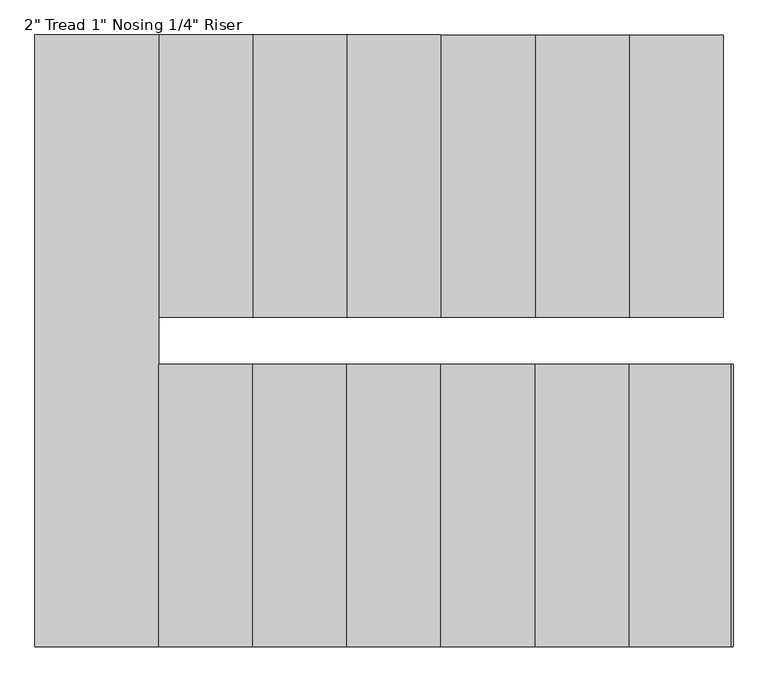
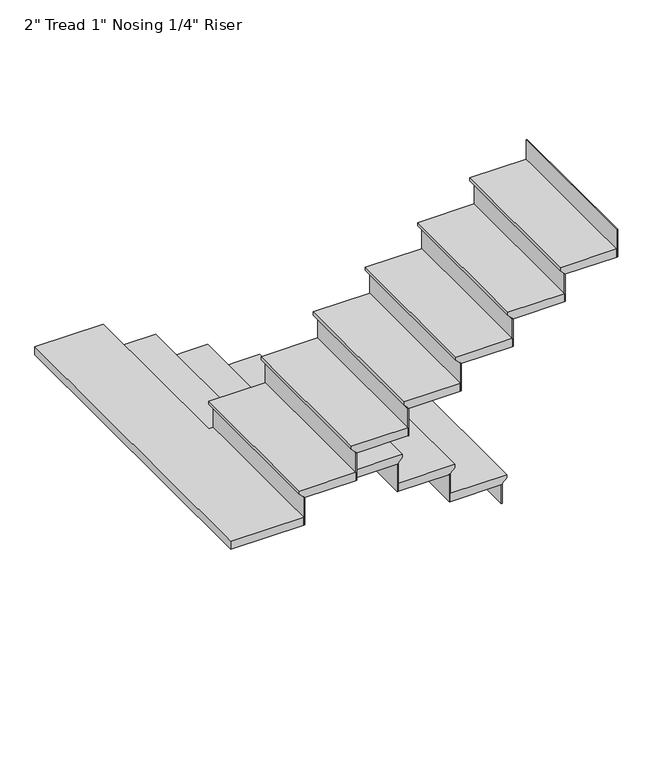
"""IFC4 building model written with IfcOpenShell, lengths in millimetres: stair flight geometry."""

from ifc_helpers import new_model, si_unit, origin, place, context, project, spatial, faceted_brep, source, transform, mapped, element, save


def stair_flight_cd429425(model_context):
    return source(origin(), model_context, "Body", "Brep", [
        faceted_brep([(3727.9146873, 3708.4, 6246.2833333), (3727.9146873, 3708.4, 6265.3333333), (3727.9146873, 2794.0, 6265.3333333), (3727.9146873, 2794.0, 6246.2833333), (3702.5146873, 3708.4, 6220.8833333), (3702.5146873, 2794.0, 6220.8833333), (3397.7146873, 3708.4, 6265.3333333), (3397.7146873, 2794.0, 6265.3333333), (3702.5146873, 2794.0, 6214.5333333), (3397.7146873, 2794.0, 6214.5333333), (3397.7146873, 3708.4, 6214.5333333), (3702.5146873, 3708.4, 6214.5333333)], [[[0, 1, 2, 3]], [[4, 0, 3, 5]], [[2, 1, 6, 7]], [[8, 9, 10, 11]], [[2, 7, 9, 8, 5, 3]], [[8, 11, 4, 5]], [[6, 1, 0, 4, 11, 10]], [[7, 6, 10, 9]]]),
        faceted_brep([(3702.5146873, 3708.4, 6214.5333333), (3702.5146873, 3708.4, 6096.0), (3696.1646873, 3708.4, 6096.0), (3696.1646873, 3708.4, 6214.5333333), (3702.5146873, 2794.0, 6214.5333333), (3696.1646873, 2794.0, 6214.5333333), (3696.1646873, 2794.0, 6096.0), (3702.5146873, 2794.0, 6096.0)], [[[0, 1, 2, 3]], [[4, 5, 6, 7]], [[1, 0, 4, 7]], [[2, 1, 7, 6]], [[3, 2, 6, 5]], [[0, 3, 5, 4]]]),
        faceted_brep([(3397.7146873, 3708.4, 6383.8666667), (3397.7146873, 3708.4, 6214.5333333), (3391.3646873, 3708.4, 6214.5333333), (3391.3646873, 3708.4, 6383.8666667), (3397.7146873, 2794.0, 6383.8666667), (3391.3646873, 2794.0, 6383.8666667), (3391.3646873, 2794.0, 6214.5333333), (3397.7146873, 2794.0, 6214.5333333)], [[[0, 1, 2, 3]], [[4, 5, 6, 7]], [[1, 0, 4, 7]], [[2, 1, 7, 6]], [[3, 2, 6, 5]], [[0, 3, 5, 4]]]),
        faceted_brep([(3423.1146873, 2794.0, 6434.6666667), (3423.1146873, 3708.4, 6434.6666667), (3092.9146873, 3708.4, 6434.6666667), (3092.9146873, 2794.0, 6434.6666667), (3397.7146873, 2794.0, 6383.8666667), (3092.9146873, 2794.0, 6383.8666667), (3092.9146873, 3708.4, 6383.8666667), (3397.7146873, 3708.4, 6383.8666667), (3397.7146873, 2794.0, 6390.2166667), (3423.1146873, 2794.0, 6415.6166667), (3397.7146873, 3708.4, 6390.2166667), (3423.1146873, 3708.4, 6415.6166667)], [[[0, 1, 2, 3]], [[4, 5, 6, 7]], [[0, 3, 5, 4, 8, 9]], [[4, 7, 10, 8]], [[2, 1, 11, 10, 7, 6]], [[3, 2, 6, 5]], [[11, 1, 0, 9]], [[10, 11, 9, 8]]]),
        faceted_brep([(3092.9146873, 3708.4, 6553.2), (3092.9146873, 3708.4, 6383.8666667), (3086.5646873, 3708.4, 6383.8666667), (3086.5646873, 3708.4, 6553.2), (3092.9146873, 2794.0, 6553.2), (3086.5646873, 2794.0, 6553.2), (3086.5646873, 2794.0, 6383.8666667), (3092.9146873, 2794.0, 6383.8666667)], [[[0, 1, 2, 3]], [[4, 5, 6, 7]], [[1, 0, 4, 7]], [[2, 1, 7, 6]], [[3, 2, 6, 5]], [[0, 3, 5, 4]]]),
        faceted_brep([(3118.3146873, 2794.0, 6604.0), (3118.3146873, 3708.4, 6604.0), (2788.1146873, 3708.4, 6604.0), (2788.1146873, 2794.0, 6604.0), (3092.9146873, 2794.0, 6553.2), (2788.1146873, 2794.0, 6553.2), (2788.1146873, 3708.4, 6553.2), (3092.9146873, 3708.4, 6553.2), (3092.9146873, 2794.0, 6559.55), (3118.3146873, 2794.0, 6584.95), (3092.9146873, 3708.4, 6559.55), (3118.3146873, 3708.4, 6584.95)], [[[0, 1, 2, 3]], [[4, 5, 6, 7]], [[0, 3, 5, 4, 8, 9]], [[4, 7, 10, 8]], [[2, 1, 11, 10, 7, 6]], [[3, 2, 6, 5]], [[11, 1, 0, 9]], [[10, 11, 9, 8]]]),
        faceted_brep([(2788.1146873, 3708.4, 6722.5333333), (2788.1146873, 3708.4, 6553.2), (2781.7646873, 3708.4, 6553.2), (2781.7646873, 3708.4, 6722.5333333), (2788.1146873, 2794.0, 6722.5333333), (2781.7646873, 2794.0, 6722.5333333), (2781.7646873, 2794.0, 6553.2), (2788.1146873, 2794.0, 6553.2)], [[[0, 1, 2, 3]], [[4, 5, 6, 7]], [[1, 0, 4, 7]], [[2, 1, 7, 6]], [[3, 2, 6, 5]], [[0, 3, 5, 4]]]),
        faceted_brep([(2813.5146873, 2794.0, 6773.3333333), (2813.5146873, 3708.4, 6773.3333333), (2483.3146873, 3708.4, 6773.3333333), (2483.3146873, 2794.0, 6773.3333333), (2788.1146873, 2794.0, 6722.5333333), (2483.3146873, 2794.0, 6722.5333333), (2483.3146873, 3708.4, 6722.5333333), (2788.1146873, 3708.4, 6722.5333333), (2788.1146873, 2794.0, 6728.8833333), (2813.5146873, 2794.0, 6754.2833333), (2788.1146873, 3708.4, 6728.8833333), (2813.5146873, 3708.4, 6754.2833333)], [[[0, 1, 2, 3]], [[4, 5, 6, 7]], [[0, 3, 5, 4, 8, 9]], [[4, 7, 10, 8]], [[2, 1, 11, 10, 7, 6]], [[3, 2, 6, 5]], [[11, 1, 0, 9]], [[10, 11, 9, 8]]]),
        faceted_brep([(2483.3146873, 3708.4, 6891.8666667), (2483.3146873, 3708.4, 6722.5333333), (2476.9646873, 3708.4, 6722.5333333), (2476.9646873, 3708.4, 6891.8666667), (2483.3146873, 2794.0, 6891.8666667), (2476.9646873, 2794.0, 6891.8666667), (2476.9646873, 2794.0, 6722.5333333), (2483.3146873, 2794.0, 6722.5333333)], [[[0, 1, 2, 3]], [[4, 5, 6, 7]], [[1, 0, 4, 7]], [[2, 1, 7, 6]], [[3, 2, 6, 5]], [[0, 3, 5, 4]]]),
        faceted_brep([(2508.7146873, 2794.0, 6942.6666667), (2508.7146873, 3708.4, 6942.6666667), (2178.5146873, 3708.4, 6942.6666667), (2178.5146873, 2794.0, 6942.6666667), (2483.3146873, 2794.0, 6891.8666667), (2178.5146873, 2794.0, 6891.8666667), (2178.5146873, 3708.4, 6891.8666667), (2483.3146873, 3708.4, 6891.8666667), (2483.3146873, 2794.0, 6898.2166667), (2508.7146873, 2794.0, 6923.6166667), (2483.3146873, 3708.4, 6898.2166667), (2508.7146873, 3708.4, 6923.6166667)], [[[0, 1, 2, 3]], [[4, 5, 6, 7]], [[0, 3, 5, 4, 8, 9]], [[4, 7, 10, 8]], [[2, 1, 11, 10, 7, 6]], [[3, 2, 6, 5]], [[11, 1, 0, 9]], [[10, 11, 9, 8]]]),
        faceted_brep([(2178.5146873, 3708.4, 7061.2), (2178.5146873, 3708.4, 6891.8666667), (2172.1646873, 3708.4, 6891.8666667), (2172.1646873, 3708.4, 7061.2), (2178.5146873, 2794.0, 7061.2), (2172.1646873, 2794.0, 7061.2), (2172.1646873, 2794.0, 6891.8666667), (2178.5146873, 2794.0, 6891.8666667)], [[[0, 1, 2, 3]], [[4, 5, 6, 7]], [[1, 0, 4, 7]], [[2, 1, 7, 6]], [[3, 2, 6, 5]], [[0, 3, 5, 4]]]),
        faceted_brep([(2203.9146873, 2794.0, 7112.0), (2203.9146873, 3708.4, 7112.0), (1873.7146873, 3708.4, 7112.0), (1873.7146873, 2794.0, 7112.0), (2178.5146873, 2794.0, 7061.2), (1873.7146873, 2794.0, 7061.2), (1873.7146873, 3708.4, 7061.2), (2178.5146873, 3708.4, 7061.2), (2178.5146873, 2794.0, 7067.55), (2203.9146873, 2794.0, 7092.95), (2178.5146873, 3708.4, 7067.55), (2203.9146873, 3708.4, 7092.95)], [[[0, 1, 2, 3]], [[4, 5, 6, 7]], [[0, 3, 5, 4, 8, 9]], [[4, 7, 10, 8]], [[2, 1, 11, 10, 7, 6]], [[3, 2, 6, 5]], [[11, 1, 0, 9]], [[10, 11, 9, 8]]]),
        faceted_brep([(1873.7146873, 3708.4, 7230.5333333), (1873.7146873, 3708.4, 7061.2), (1867.3646873, 3708.4, 7061.2), (1867.3646873, 3708.4, 7230.5333333), (1873.7146873, 2794.0, 7230.5333333), (1867.3646873, 2794.0, 7230.5333333), (1867.3646873, 2794.0, 7061.2), (1873.7146873, 2794.0, 7061.2)], [[[0, 1, 2, 3]], [[4, 5, 6, 7]], [[1, 0, 4, 7]], [[2, 1, 7, 6]], [[3, 2, 6, 5]], [[0, 3, 5, 4]]]),
        faceted_brep([(1924.5146873, 2641.6, 7281.3333333), (1899.1146873, 2641.6, 7281.3333333), (1899.1146873, 3708.4, 7281.3333333), (1498.6, 3708.4, 7281.3333333), (1498.6, 1727.2, 7281.3333333), (1924.5146873, 1727.2, 7281.3333333), (1899.1146873, 2641.6, 7230.5333333), (1924.5146873, 2641.6, 7230.5333333), (1924.5146873, 1727.2, 7230.5333333), (1498.6, 1727.2, 7230.5333333), (1498.6, 3708.4, 7230.5333333), (1873.7146873, 3708.4, 7230.5333333), (1873.7146873, 2794.0, 7230.5333333), (1899.1146873, 2794.0, 7230.5333333), (1899.1146873, 2794.0, 7262.2833333), (1899.1146873, 3708.4, 7262.2833333), (1873.7146873, 2794.0, 7236.8833333), (1873.7146873, 3708.4, 7236.8833333)], [[[0, 1, 2, 3, 4, 5]], [[6, 7, 8, 9, 10, 11, 12, 13]], [[1, 0, 7, 6]], [[2, 1, 6, 13, 14, 15]], [[13, 12, 16, 14]], [[12, 11, 17, 16]], [[3, 2, 15, 17, 11, 10]], [[4, 3, 10, 9]], [[5, 4, 9, 8]], [[0, 5, 8, 7]], [[17, 15, 14, 16]]]),
        faceted_brep([(1924.5146873, 1727.2, 7399.8666667), (1924.5146873, 1727.2, 7230.5333333), (1930.8646873, 1727.2, 7230.5333333), (1930.8646873, 1727.2, 7399.8666667), (1924.5146873, 2641.6, 7399.8666667), (1930.8646873, 2641.6, 7399.8666667), (1930.8646873, 2641.6, 7230.5333333), (1924.5146873, 2641.6, 7230.5333333)], [[[0, 1, 2, 3]], [[4, 5, 6, 7]], [[1, 0, 4, 7]], [[2, 1, 7, 6]], [[3, 2, 6, 5]], [[0, 3, 5, 4]]]),
        faceted_brep([(1899.1146873, 2641.6, 7450.6666667), (1899.1146873, 1727.2, 7450.6666667), (2229.3146873, 1727.2, 7450.6666667), (2229.3146873, 2641.6, 7450.6666667), (1924.5146873, 2641.6, 7399.8666667), (2229.3146873, 2641.6, 7399.8666667), (2229.3146873, 1727.2, 7399.8666667), (1924.5146873, 1727.2, 7399.8666667), (1924.5146873, 2641.6, 7406.2166667), (1899.1146873, 2641.6, 7431.6166667), (1924.5146873, 1727.2, 7406.2166667), (1899.1146873, 1727.2, 7431.6166667)], [[[0, 1, 2, 3]], [[4, 5, 6, 7]], [[0, 3, 5, 4, 8, 9]], [[4, 7, 10, 8]], [[2, 1, 11, 10, 7, 6]], [[3, 2, 6, 5]], [[11, 1, 0, 9]], [[10, 11, 9, 8]]]),
        faceted_brep([(2229.3146873, 1727.2, 7569.2), (2229.3146873, 1727.2, 7399.8666667), (2235.6646873, 1727.2, 7399.8666667), (2235.6646873, 1727.2, 7569.2), (2229.3146873, 2641.6, 7569.2), (2235.6646873, 2641.6, 7569.2), (2235.6646873, 2641.6, 7399.8666667), (2229.3146873, 2641.6, 7399.8666667)], [[[0, 1, 2, 3]], [[4, 5, 6, 7]], [[1, 0, 4, 7]], [[2, 1, 7, 6]], [[3, 2, 6, 5]], [[0, 3, 5, 4]]]),
        faceted_brep([(2203.9146873, 2641.6, 7620.0), (2203.9146873, 1727.2, 7620.0), (2534.1146873, 1727.2, 7620.0), (2534.1146873, 2641.6, 7620.0), (2229.3146873, 2641.6, 7569.2), (2534.1146873, 2641.6, 7569.2), (2534.1146873, 1727.2, 7569.2), (2229.3146873, 1727.2, 7569.2), (2229.3146873, 2641.6, 7575.55), (2203.9146873, 2641.6, 7600.95), (2229.3146873, 1727.2, 7575.55), (2203.9146873, 1727.2, 7600.95)], [[[0, 1, 2, 3]], [[4, 5, 6, 7]], [[0, 3, 5, 4, 8, 9]], [[4, 7, 10, 8]], [[2, 1, 11, 10, 7, 6]], [[3, 2, 6, 5]], [[11, 1, 0, 9]], [[10, 11, 9, 8]]]),
        faceted_brep([(2534.1146873, 1727.2, 7738.5333333), (2534.1146873, 1727.2, 7569.2), (2540.4646873, 1727.2, 7569.2), (2540.4646873, 1727.2, 7738.5333333), (2534.1146873, 2641.6, 7738.5333333), (2540.4646873, 2641.6, 7738.5333333), (2540.4646873, 2641.6, 7569.2), (2534.1146873, 2641.6, 7569.2)], [[[0, 1, 2, 3]], [[4, 5, 6, 7]], [[1, 0, 4, 7]], [[2, 1, 7, 6]], [[3, 2, 6, 5]], [[0, 3, 5, 4]]]),
        faceted_brep([(2508.7146873, 2641.6, 7789.3333333), (2508.7146873, 1727.2, 7789.3333333), (2838.9146873, 1727.2, 7789.3333333), (2838.9146873, 2641.6, 7789.3333333), (2534.1146873, 2641.6, 7738.5333333), (2838.9146873, 2641.6, 7738.5333333), (2838.9146873, 1727.2, 7738.5333333), (2534.1146873, 1727.2, 7738.5333333), (2534.1146873, 2641.6, 7744.8833333), (2508.7146873, 2641.6, 7770.2833333), (2534.1146873, 1727.2, 7744.8833333), (2508.7146873, 1727.2, 7770.2833333)], [[[0, 1, 2, 3]], [[4, 5, 6, 7]], [[0, 3, 5, 4, 8, 9]], [[4, 7, 10, 8]], [[2, 1, 11, 10, 7, 6]], [[3, 2, 6, 5]], [[11, 1, 0, 9]], [[10, 11, 9, 8]]]),
        faceted_brep([(2838.9146873, 1727.2, 7907.8666667), (2838.9146873, 1727.2, 7738.5333333), (2845.2646873, 1727.2, 7738.5333333), (2845.2646873, 1727.2, 7907.8666667), (2838.9146873, 2641.6, 7907.8666667), (2845.2646873, 2641.6, 7907.8666667), (2845.2646873, 2641.6, 7738.5333333), (2838.9146873, 2641.6, 7738.5333333)], [[[0, 1, 2, 3]], [[4, 5, 6, 7]], [[1, 0, 4, 7]], [[2, 1, 7, 6]], [[3, 2, 6, 5]], [[0, 3, 5, 4]]]),
        faceted_brep([(2813.5146873, 2641.6, 7958.6666667), (2813.5146873, 1727.2, 7958.6666667), (3143.7146873, 1727.2, 7958.6666667), (3143.7146873, 2641.6, 7958.6666667), (2838.9146873, 2641.6, 7907.8666667), (3143.7146873, 2641.6, 7907.8666667), (3143.7146873, 1727.2, 7907.8666667), (2838.9146873, 1727.2, 7907.8666667), (2838.9146873, 2641.6, 7914.2166667), (2813.5146873, 2641.6, 7939.6166667), (2838.9146873, 1727.2, 7914.2166667), (2813.5146873, 1727.2, 7939.6166667)], [[[0, 1, 2, 3]], [[4, 5, 6, 7]], [[0, 3, 5, 4, 8, 9]], [[4, 7, 10, 8]], [[2, 1, 11, 10, 7, 6]], [[3, 2, 6, 5]], [[11, 1, 0, 9]], [[10, 11, 9, 8]]]),
        faceted_brep([(3143.7146873, 1727.2, 8077.2), (3143.7146873, 1727.2, 7907.8666667), (3150.0646873, 1727.2, 7907.8666667), (3150.0646873, 1727.2, 8077.2), (3143.7146873, 2641.6, 8077.2), (3150.0646873, 2641.6, 8077.2), (3150.0646873, 2641.6, 7907.8666667), (3143.7146873, 2641.6, 7907.8666667)], [[[0, 1, 2, 3]], [[4, 5, 6, 7]], [[1, 0, 4, 7]], [[2, 1, 7, 6]], [[3, 2, 6, 5]], [[0, 3, 5, 4]]]),
        faceted_brep([(3118.3146873, 2641.6, 8128.0), (3118.3146873, 1727.2, 8128.0), (3448.5146873, 1727.2, 8128.0), (3448.5146873, 2641.6, 8128.0), (3143.7146873, 2641.6, 8077.2), (3448.5146873, 2641.6, 8077.2), (3448.5146873, 1727.2, 8077.2), (3143.7146873, 1727.2, 8077.2), (3143.7146873, 2641.6, 8083.55), (3118.3146873, 2641.6, 8108.95), (3143.7146873, 1727.2, 8083.55), (3118.3146873, 1727.2, 8108.95)], [[[0, 1, 2, 3]], [[4, 5, 6, 7]], [[0, 3, 5, 4, 8, 9]], [[4, 7, 10, 8]], [[2, 1, 11, 10, 7, 6]], [[3, 2, 6, 5]], [[11, 1, 0, 9]], [[10, 11, 9, 8]]]),
        faceted_brep([(3448.5146873, 1727.2, 8246.5333333), (3448.5146873, 1727.2, 8077.2), (3454.8646873, 1727.2, 8077.2), (3454.8646873, 1727.2, 8246.5333333), (3448.5146873, 2641.6, 8246.5333333), (3454.8646873, 2641.6, 8246.5333333), (3454.8646873, 2641.6, 8077.2), (3448.5146873, 2641.6, 8077.2)], [[[0, 1, 2, 3]], [[4, 5, 6, 7]], [[1, 0, 4, 7]], [[2, 1, 7, 6]], [[3, 2, 6, 5]], [[0, 3, 5, 4]]]),
        faceted_brep([(3753.3146873, 1727.2, 8415.8666667), (3753.3146873, 1727.2, 8246.5333333), (3759.6646873, 1727.2, 8246.5333333), (3759.6646873, 1727.2, 8415.8666667), (3753.3146873, 2641.6, 8415.8666667), (3759.6646873, 2641.6, 8415.8666667), (3759.6646873, 2641.6, 8246.5333333), (3753.3146873, 2641.6, 8246.5333333)], [[[0, 1, 2, 3]], [[4, 5, 6, 7]], [[1, 0, 4, 7]], [[2, 1, 7, 6]], [[3, 2, 6, 5]], [[0, 3, 5, 4]]]),
        faceted_brep([(3423.1146873, 2641.6, 8297.3333333), (3423.1146873, 1727.2, 8297.3333333), (3753.3146873, 1727.2, 8297.3333333), (3753.3146873, 2641.6, 8297.3333333), (3448.5146873, 2641.6, 8246.5333333), (3753.3146873, 2641.6, 8246.5333333), (3753.3146873, 1727.2, 8246.5333333), (3448.5146873, 1727.2, 8246.5333333), (3448.5146873, 2641.6, 8252.8833333), (3423.1146873, 2641.6, 8278.2833333), (3448.5146873, 1727.2, 8252.8833333), (3423.1146873, 1727.2, 8278.2833333)], [[[0, 1, 2, 3]], [[4, 5, 6, 7]], [[0, 3, 5, 4, 8, 9]], [[4, 7, 10, 8]], [[2, 1, 11, 10, 7, 6]], [[3, 2, 6, 5]], [[11, 1, 0, 9]], [[10, 11, 9, 8]]]),
    ])


if __name__ == "__main__":
    model = new_model("IFC4")
    model_context = context("Model", 3, world=origin())
    ifc_project = project(units=[si_unit("LENGTHUNIT", "METRE", prefix="MILLI")], contexts=[model_context])
    site = spatial("IfcSite", under=ifc_project)
    building = spatial("IfcBuilding", under=site)
    placement = place(None, origin())
    stair_flight_shape = stair_flight_cd429425(model_context)
    element("IfcStairFlight", 1, ObjectType="2\" Tread 1\" Nosing 1/4\" Riser", at=placement, inside=building, context=model_context, shape_type="MappedRepresentation", body=[
        mapped(stair_flight_shape, transform((0.0, 0.0, 0.0), x_axis=(1.0, 0.0, 0.0), y_axis=(0.0, 1.0, 0.0), z_axis=(0.0, 0.0, 1.0))),
    ])
    save(model, "model.ifc")
